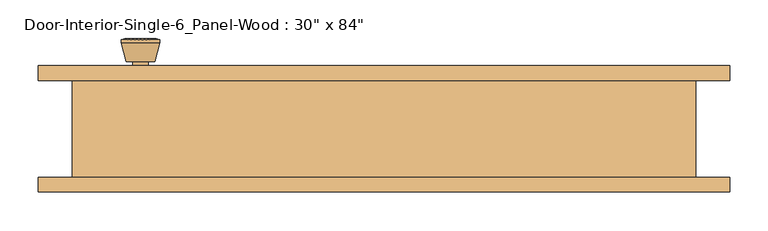
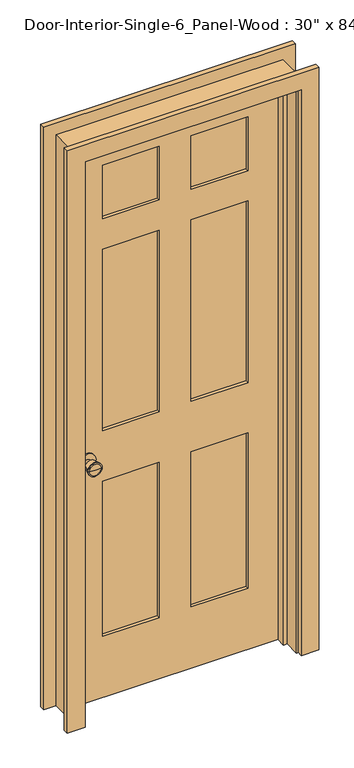
"""IFC4 building model written with IfcOpenShell, lengths in millimetres: door geometry."""

from ifc_helpers import new_model, si_unit, point, frame, frame_2d, origin, place, context, project, spatial, polyline, circle_curve, trimmed, segment, composite_curve, outline, extrude, faceted_brep, source, transform, mapped, element, save
from ifc_brep_helpers import plane_surface, cylinder_surface, revolved_surface, advanced_brep


def door_d66ee888(model_context):
    return source(origin(), model_context, "Body", "SolidModel", [
        advanced_brep(
        [(-317.5, 19.4, 914.4), (-307.5, 19.4, 914.4), (-327.5, 19.4, 914.4), (-297.0241324, -29.6, 914.4), (-317.5, -29.6, 914.4), (-337.9758676, -29.6, 914.4), (-292.5, -27.7721319, 914.4), (-342.5, -27.7721319, 914.4), (-292.5, -24.3084537, 914.4), (-342.5, -24.3084537, 914.4), (-298.863764, 0.4, 914.4), (-336.136236, 0.4, 914.4), (-307.5, 0.4, 914.4), (-327.5, 0.4, 914.4)],
        [
            (0, 1),
            (1, 2, circle_curve(frame((-317.5, 19.4, 914.4), z_axis=(0.0, 1.0, 0.0), x_axis=(-1.0, 0.0, 0.0)), 10.0)),
            (2, 0),
            (2, 1, circle_curve(frame((-317.5, 19.4, 914.4), z_axis=(0.0, 1.0, 0.0), x_axis=(-1.0, 0.0, 0.0)), 10.0)),
            (3, 4),
            (4, 5),
            (5, 3, circle_curve(frame((-317.5, -29.6, 914.4), z_axis=(0.0, -1.0, 0.0), x_axis=(-1.0, 0.0, 0.0)), 20.4758676)),
            (3, 5, circle_curve(frame((-317.5, -29.6, 914.4), z_axis=(0.0, -1.0, 0.0), x_axis=(-1.0, 0.0, 0.0)), 20.4758676)),
            (6, 3),
            (5, 7),
            (7, 6, circle_curve(frame((-317.5, -27.7721319, 914.4), z_axis=(0.0, -1.0, 0.0), x_axis=(-1.0, 0.0, 0.0)), 25.0)),
            (6, 7, circle_curve(frame((-317.5, -27.7721319, 914.4), z_axis=(0.0, -1.0, 0.0), x_axis=(-1.0, 0.0, 0.0)), 25.0)),
            (8, 6),
            (7, 9),
            (9, 8, circle_curve(frame((-317.5, -24.3084537, 914.4), z_axis=(0.0, -1.0, 0.0), x_axis=(-1.0, 0.0, 0.0)), 25.0)),
            (8, 9, circle_curve(frame((-317.5, -24.3084537, 914.4), z_axis=(0.0, -1.0, 0.0), x_axis=(-1.0, 0.0, 0.0)), 25.0)),
            (10, 8),
            (9, 11),
            (11, 10, circle_curve(frame((-317.5, 0.4, 914.4), z_axis=(0.0, -1.0, 0.0), x_axis=(-1.0, 0.0, 0.0)), 18.636236)),
            (10, 11, circle_curve(frame((-317.5, 0.4, 914.4), z_axis=(0.0, -1.0, 0.0), x_axis=(-1.0, 0.0, 0.0)), 18.636236)),
            (12, 10),
            (11, 13),
            (13, 12, circle_curve(frame((-317.5, 0.4, 914.4), z_axis=(0.0, -1.0, 0.0), x_axis=(-1.0, 0.0, 0.0)), 10.0)),
            (12, 13, circle_curve(frame((-317.5, 0.4, 914.4), z_axis=(0.0, -1.0, 0.0), x_axis=(-1.0, 0.0, 0.0)), 10.0)),
            (1, 12),
            (13, 2),
        ],
        [
            plane_surface(frame((-317.5, 19.4, 914.4), z_axis=(0.0, 1.0, 0.0), x_axis=(-1.0, 0.0, 0.0))),
            plane_surface(frame((-317.5, -29.6, 914.4), z_axis=(0.0, -1.0, 0.0), x_axis=(-1.0, 0.0, 0.0))),
            revolved_surface(polyline([(-337.9758676, -29.6, 914.4), (-342.5, -27.7721319, 914.4)]), (-317.5, 19.4, 914.4), (0.0, 1.0, 0.0)),
            cylinder_surface(frame((-317.5, 19.4, 914.4), z_axis=(0.0, 1.0, 0.0), x_axis=(-1.0, 0.0, 0.0)), 25.0),
            revolved_surface(polyline([(-342.5, -24.3084537, 914.4), (-336.136236, 0.4, 914.4)]), (-317.5, 19.4, 914.4), (0.0, 1.0, 0.0)),
            plane_surface(frame((-317.5, 0.4, 914.4), z_axis=(0.0, 1.0, 0.0), x_axis=(-1.0, 0.0, 0.0))),
            cylinder_surface(frame((-317.5, 19.4, 914.4), z_axis=(0.0, 1.0, 0.0), x_axis=(-1.0, 0.0, 0.0)), 10.0),
        ],
        [
            (0, [[1, 2, 3]]),
            (0, [[-3, 4, -1]]),
            (1, [[5, 6, 7]]),
            (1, [[-6, -5, 8]]),
            (2, [[9, -7, 10, 11]]),
            (2, [[-10, -8, -9, 12]]),
            (3, [[13, -11, 14, 15]]),
            (3, [[-14, -12, -13, 16]]),
            (4, [[17, -15, 18, 19]]),
            (4, [[-18, -16, -17, 20]]),
            (5, [[21, -19, 22, 23]]),
            (5, [[-22, -20, -21, 24]]),
            (6, [[25, -23, 26, -2]]),
            (6, [[-26, -24, -25, -4]]),
        ],
    ),
        extrude(outline(composite_curve([segment(trimmed(circle_curve(frame_2d((914.4, -317.5)), 30.0), [point((914.4, -347.5))], [point((914.4, -287.5))], False, "CARTESIAN"), True, "CONTINUOUS"), segment(trimmed(circle_curve(frame_2d((914.4, -317.5)), 30.0), [point((914.4, -287.5))], [point((914.4, -347.5))], False, "CARTESIAN"), True, "CONTINUOUS")], self_intersect=False)), frame((0.0, 19.4, 0.0), z_axis=(0.0, 1.0, 0.0), x_axis=(0.0, 0.0, 1.0)), (0.0, 0.0, 1.0), 6.0),
        advanced_brep(
        [(-317.5, 66.325, 914.4), (-327.5, 66.325, 914.4), (-307.5, 66.325, 914.4), (-297.0241324, 115.325, 914.4), (-337.9758676, 115.325, 914.4), (-317.5, 115.325, 914.4), (-292.5, 113.4971319, 914.4), (-342.5, 113.4971319, 914.4), (-292.5, 110.0334537, 914.4), (-342.5, 110.0334537, 914.4), (-298.863764, 85.325, 914.4), (-336.136236, 85.325, 914.4), (-307.5, 85.325, 914.4), (-327.5, 85.325, 914.4)],
        [
            (0, 1),
            (1, 2, circle_curve(frame((-317.5, 66.325, 914.4), z_axis=(0.0, -1.0, 0.0), x_axis=(-1.0, 0.0, 0.0)), 10.0)),
            (2, 0),
            (2, 1, circle_curve(frame((-317.5, 66.325, 914.4), z_axis=(0.0, -1.0, 0.0), x_axis=(-1.0, 0.0, 0.0)), 10.0)),
            (3, 4, circle_curve(frame((-317.5, 115.325, 914.4), z_axis=(0.0, 1.0, 0.0), x_axis=(-1.0, 0.0, 0.0)), 20.4758676)),
            (4, 5),
            (5, 3),
            (4, 3, circle_curve(frame((-317.5, 115.325, 914.4), z_axis=(0.0, 1.0, 0.0), x_axis=(-1.0, 0.0, 0.0)), 20.4758676)),
            (6, 7, circle_curve(frame((-317.5, 113.4971319, 914.4), z_axis=(0.0, 1.0, 0.0), x_axis=(-1.0, 0.0, 0.0)), 25.0)),
            (7, 4),
            (3, 6),
            (7, 6, circle_curve(frame((-317.5, 113.4971319, 914.4), z_axis=(0.0, 1.0, 0.0), x_axis=(-1.0, 0.0, 0.0)), 25.0)),
            (8, 9, circle_curve(frame((-317.5, 110.0334537, 914.4), z_axis=(0.0, 1.0, 0.0), x_axis=(-1.0, 0.0, 0.0)), 25.0)),
            (9, 7),
            (6, 8),
            (9, 8, circle_curve(frame((-317.5, 110.0334537, 914.4), z_axis=(0.0, 1.0, 0.0), x_axis=(-1.0, 0.0, 0.0)), 25.0)),
            (10, 11, circle_curve(frame((-317.5, 85.325, 914.4), z_axis=(0.0, 1.0, 0.0), x_axis=(-1.0, 0.0, 0.0)), 18.636236)),
            (11, 9),
            (8, 10),
            (11, 10, circle_curve(frame((-317.5, 85.325, 914.4), z_axis=(0.0, 1.0, 0.0), x_axis=(-1.0, 0.0, 0.0)), 18.636236)),
            (12, 13, circle_curve(frame((-317.5, 85.325, 914.4), z_axis=(0.0, 1.0, 0.0), x_axis=(-1.0, 0.0, 0.0)), 10.0)),
            (13, 11),
            (10, 12),
            (13, 12, circle_curve(frame((-317.5, 85.325, 914.4), z_axis=(0.0, 1.0, 0.0), x_axis=(-1.0, 0.0, 0.0)), 10.0)),
            (1, 13),
            (12, 2),
        ],
        [
            plane_surface(frame((-317.5, 66.325, 914.4), z_axis=(0.0, -1.0, 0.0), x_axis=(-1.0, 0.0, 0.0))),
            plane_surface(frame((-317.5, 115.325, 914.4), z_axis=(0.0, 1.0, 0.0), x_axis=(-1.0, 0.0, 0.0))),
            revolved_surface(polyline([(-337.9758676, 115.325, 914.4), (-342.5, 113.4971319, 914.4)]), (-317.5, 66.325, 914.4), (0.0, -1.0, 0.0)),
            cylinder_surface(frame((-317.5, 66.325, 914.4), z_axis=(0.0, -1.0, 0.0), x_axis=(-1.0, 0.0, 0.0)), 25.0),
            revolved_surface(polyline([(-342.5, 110.0334537, 914.4), (-336.136236, 85.325, 914.4)]), (-317.5, 66.325, 914.4), (0.0, -1.0, 0.0)),
            plane_surface(frame((-317.5, 85.325, 914.4), z_axis=(0.0, -1.0, 0.0), x_axis=(-1.0, 0.0, 0.0))),
            cylinder_surface(frame((-317.5, 66.325, 914.4), z_axis=(0.0, -1.0, 0.0), x_axis=(-1.0, 0.0, 0.0)), 10.0),
        ],
        [
            (0, [[1, 2, 3]]),
            (0, [[-3, 4, -1]]),
            (1, [[5, 6, 7]]),
            (1, [[8, -7, -6]]),
            (2, [[9, 10, -5, 11]]),
            (2, [[12, -11, -8, -10]]),
            (3, [[13, 14, -9, 15]]),
            (3, [[16, -15, -12, -14]]),
            (4, [[17, 18, -13, 19]]),
            (4, [[20, -19, -16, -18]]),
            (5, [[21, 22, -17, 23]]),
            (5, [[24, -23, -20, -22]]),
            (6, [[-2, 25, -21, 26]]),
            (6, [[-4, -26, -24, -25]]),
        ],
    ),
        extrude(outline(composite_curve([segment(trimmed(circle_curve(frame_2d((914.4, -317.5)), 30.0), [point((914.4, -347.5))], [point((914.4, -287.5))], False, "CARTESIAN"), True, "CONTINUOUS"), segment(trimmed(circle_curve(frame_2d((914.4, -317.5)), 30.0), [point((914.4, -287.5))], [point((914.4, -347.5))], False, "CARTESIAN"), True, "CONTINUOUS")], self_intersect=False)), frame((0.0, 60.325, 0.0), z_axis=(0.0, 1.0, 0.0), x_axis=(0.0, 0.0, 1.0)), (0.0, 0.0, 1.0), 6.0),
        faceted_brep([(406.4, 60.325, 0.0), (406.4, -66.675, 0.0), (381.0, -66.675, 0.0), (381.0, -9.525, 0.0), (368.3, -9.525, 0.0), (368.3, 25.4, 0.0), (381.0, 25.4, 0.0), (381.0, 60.325, 0.0), (406.4, 60.325, 2159.0), (406.4, -66.675, 2159.0), (-406.4, -66.675, 2159.0), (-406.4, -66.675, 0.0), (-381.0, -66.675, 0.0), (-381.0, -66.675, 2133.6), (381.0, -66.675, 2133.6), (381.0, -9.525, 2133.6), (-381.0, -9.525, 2133.6), (-381.0, -9.525, 0.0), (-368.3, -9.525, 0.0), (-368.3, -9.525, 2120.9), (368.3, -9.525, 2120.9), (368.3, 25.4, 2120.9), (-368.3, 25.4, 2120.9), (-368.3, 25.4, 0.0), (-381.0, 25.4, 0.0), (-381.0, 25.4, 2133.6), (381.0, 25.4, 2133.6), (381.0, 60.325, 2133.6), (-381.0, 60.325, 2133.6), (-381.0, 60.325, 0.0), (-406.4, 60.325, 0.0), (-406.4, 60.325, 2159.0)], [[[0, 1, 2, 3, 4, 5, 6, 7]], [[1, 0, 8, 9]], [[2, 1, 9, 10, 11, 12, 13, 14]], [[3, 2, 14, 15]], [[4, 3, 15, 16, 17, 18, 19, 20]], [[5, 4, 20, 21]], [[6, 5, 21, 22, 23, 24, 25, 26]], [[7, 6, 26, 27]], [[0, 7, 27, 28, 29, 30, 31, 8]], [[9, 8, 31, 10]], [[15, 14, 13, 16]], [[21, 20, 19, 22]], [[27, 26, 25, 28]], [[30, 29, 24, 23, 18, 17, 12, 11]], [[10, 31, 30, 11]], [[16, 13, 12, 17]], [[22, 19, 18, 23]], [[28, 25, 24, 29]]]),
        extrude(outline(polyline([(2133.6, -381.0), (0.0, -381.0), (0.0, 381.0), (2133.6, 381.0), (2133.6, -381.0)]), holes=[polyline([(2014.5375, 57.15), (2014.5375, 260.35), (1811.3375, 260.35), (1811.3375, 57.15), (2014.5375, 57.15)]), polyline([(1697.0375, 260.35), (1009.65, 260.35), (1009.65, 57.15), (1697.0375, 57.15), (1697.0375, 260.35)]), polyline([(1009.65, -57.15), (1009.65, -260.35), (1697.0375, -260.35), (1697.0375, -57.15), (1009.65, -57.15)]), polyline([(1811.3375, -260.35), (2014.5375, -260.35), (2014.5375, -57.15), (1811.3375, -57.15), (1811.3375, -260.35)]), polyline([(819.15, 57.15), (819.15, 260.35), (231.775, 260.35), (231.775, 57.15), (819.15, 57.15)]), polyline([(231.775, -57.15), (231.775, -260.35), (819.15, -260.35), (819.15, -57.15), (231.775, -57.15)])]), frame((0.0, 25.4, 0.0), z_axis=(0.0, 1.0, 0.0), x_axis=(0.0, 0.0, 1.0)), (0.0, 0.0, 1.0), 34.925),
        extrude(outline(polyline([(260.35, 37.0416667), (57.15, 37.0416667), (57.15, 48.6833333), (260.35, 48.6833333), (260.35, 37.0416667)])), frame((0.0, 0.0, 1811.3375), z_axis=(0.0, 0.0, 1.0), x_axis=(1.0, 0.0, 0.0)), (0.0, 0.0, 1.0), 203.2),
        extrude(outline(polyline([(260.35, 37.0416667), (57.15, 37.0416667), (57.15, 48.6833333), (260.35, 48.6833333), (260.35, 37.0416667)])), frame((0.0, 0.0, 1009.65), z_axis=(0.0, 0.0, 1.0), x_axis=(1.0, 0.0, 0.0)), (0.0, 0.0, 1.0), 687.3875),
        extrude(outline(polyline([(-57.15, 37.0416667), (-260.35, 37.0416667), (-260.35, 48.6833333), (-57.15, 48.6833333), (-57.15, 37.0416667)])), frame((0.0, 0.0, 1009.65), z_axis=(0.0, 0.0, 1.0), x_axis=(1.0, 0.0, 0.0)), (0.0, 0.0, 1.0), 687.3875),
        extrude(outline(polyline([(-57.15, 37.0416667), (-260.35, 37.0416667), (-260.35, 48.6833333), (-57.15, 48.6833333), (-57.15, 37.0416667)])), frame((0.0, 0.0, 1811.3375), z_axis=(0.0, 0.0, 1.0), x_axis=(1.0, 0.0, 0.0)), (0.0, 0.0, 1.0), 203.2),
        extrude(outline(polyline([(260.35, 37.0416667), (57.15, 37.0416667), (57.15, 48.6833333), (260.35, 48.6833333), (260.35, 37.0416667)])), frame((0.0, 0.0, 231.775), z_axis=(0.0, 0.0, 1.0), x_axis=(1.0, 0.0, 0.0)), (0.0, 0.0, 1.0), 587.375),
        extrude(outline(polyline([(-57.15, 37.0416667), (-260.35, 37.0416667), (-260.35, 48.6833333), (-57.15, 48.6833333), (-57.15, 37.0416667)])), frame((0.0, 0.0, 231.775), z_axis=(0.0, 0.0, 1.0), x_axis=(1.0, 0.0, 0.0)), (0.0, 0.0, 1.0), 587.375),
        extrude(outline(polyline([(0.0, 387.35), (0.0, 450.85), (2203.45, 450.85), (2203.45, -450.85), (0.0, -450.85), (0.0, -387.35), (2139.95, -387.35), (2139.95, 387.35), (0.0, 387.35)])), frame((0.0, 60.325, 0.0), z_axis=(0.0, 1.0, 0.0), x_axis=(0.0, 0.0, 1.0)), (0.0, 0.0, 1.0), 19.05),
        extrude(outline(polyline([(0.0, 387.35), (0.0, 450.85), (2203.45, 450.85), (2203.45, -450.85), (0.0, -450.85), (0.0, -387.35), (2139.95, -387.35), (2139.95, 387.35), (0.0, 387.35)])), frame((0.0, -85.725, 0.0), z_axis=(0.0, 1.0, 0.0), x_axis=(0.0, 0.0, 1.0)), (0.0, 0.0, 1.0), 19.05),
    ])


if __name__ == "__main__":
    model = new_model("IFC4")
    model_context = context("Model", 3, world=origin())
    ifc_project = project(units=[si_unit("LENGTHUNIT", "METRE", prefix="MILLI")], contexts=[model_context])
    site = spatial("IfcSite", under=ifc_project)
    building = spatial("IfcBuilding", under=site)
    placement = place(None, origin())
    door_shape = door_d66ee888(model_context)
    element("IfcDoor", 1, ObjectType="Door-Interior-Single-6_Panel-Wood : 30\" x 84\"", at=placement, inside=building, context=model_context, shape_type="MappedRepresentation", body=[
        mapped(door_shape, transform((0.0, 0.0, 0.0), x_axis=(1.0, 0.0, 0.0), y_axis=(0.0, 1.0, 0.0), z_axis=(0.0, 0.0, 1.0))),
    ])
    save(model, "model.ifc")

# Revit data of these elements
# Type "Door-Interior-Single-6_Panel-Wood : 30\" x 84\""
#   Type Mark = "9"
#   Assembly Code = "C1020300"
#   Analytic Construction = "Wooden"
#   Top Rail = 0' - 4 11/16"
#   Top Panel = 0' - 8"
#   Thickness = 0' - 1 3/8"
#   Thermal Resistance (R) = 2.5876 (h·ft²·°F)/BTU
#   Swing Angle [instance default] = 90.00°
#   Stiles = 0' - 4 3/4"
#   Rough Width = 2' - 8"
#   Rough Height = 7' - 1"
#   Mullion = 0' - 4 1/2"
#   Lock Rail = 0' - 7 1/2"
#   Intermediate Rail = 0' - 4 1/2"
#   Height = 7' - 0"
#   Width = 2' - 6"
#   Heat Transfer Coefficient (U) = 0.3865 BTU/(h·ft²·°F)
#   Bottom Rail = 0' - 9 1/8"
#   Trim Material = Cherry
#   Panel Material = Cherry
#   Frame Material = Cherry
#   Door Handle Material = Aluminum
#   Visual Light Transmittance = 0
#   Solar Heat Gain Coefficient = 0
#   Wall Closure = (empty or 0)
#   Function = (empty or 0)
# Element 1 (IfcDoor, "Door-Interior-Single-6_Panel-Wood : 30\" x 84\"")
#   Materials on its faces: "Cherry", "Aluminum"
# Materials
#   "Cherry": class "Wood", colour RGB 226 177 128, transparency 0, Description = "Prunus Serotina", Cost = 0
#   "Aluminum": class "Metal", colour RGB 247 247 247, transparency 0, Description = "Aluminum 6061", Cost = 0
